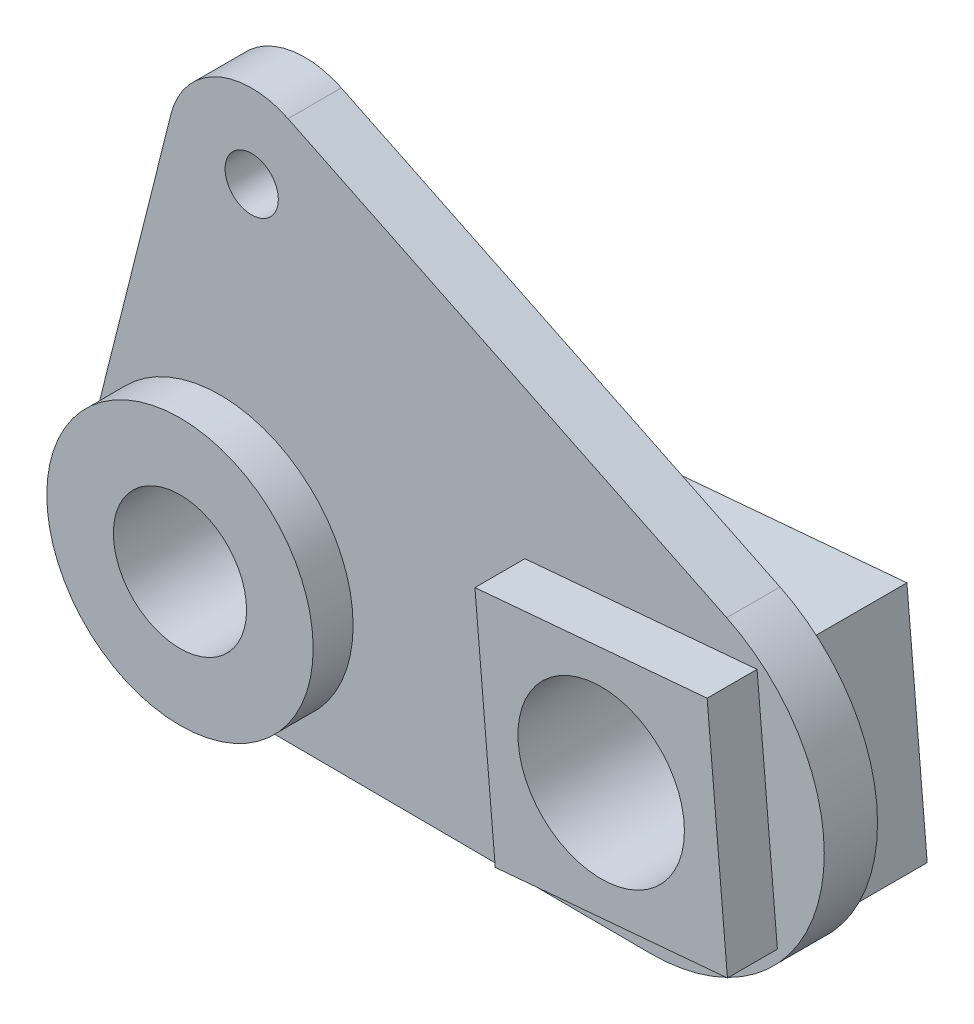
ISO-10303-21;
HEADER;
FILE_DESCRIPTION(('STEP AP214'),'2;1');
FILE_NAME('part.step','',(''),(''),'','','');
FILE_SCHEMA(('AUTOMOTIVE_DESIGN { 1 0 10303 214 1 1 1 1 }'));
ENDSEC;
DATA;
#1=APPLICATION_CONTEXT('core data for automotive mechanical design processes');
#2=APPLICATION_PROTOCOL_DEFINITION('international standard','automotive_design',2000,#1);
#3=PRODUCT_CONTEXT('',#1,'mechanical');
#4=PRODUCT('Part','Part','',(#3));
#5=PRODUCT_RELATED_PRODUCT_CATEGORY('part','',(#4));
#6=PRODUCT_DEFINITION_FORMATION('','',#4);
#7=PRODUCT_DEFINITION_CONTEXT('part definition',#1,'design');
#8=PRODUCT_DEFINITION('design','',#6,#7);
#9=PRODUCT_DEFINITION_SHAPE('','',#8);
#10=(LENGTH_UNIT() NAMED_UNIT(*) SI_UNIT(.MILLI.,.METRE.));
#11=(NAMED_UNIT(*) PLANE_ANGLE_UNIT() SI_UNIT($,.RADIAN.));
#12=(NAMED_UNIT(*) SI_UNIT($,.STERADIAN.) SOLID_ANGLE_UNIT());
#13=UNCERTAINTY_MEASURE_WITH_UNIT(LENGTH_MEASURE(1.E-05),#10,'distance_accuracy_value','');
#14=(GEOMETRIC_REPRESENTATION_CONTEXT(3) GLOBAL_UNCERTAINTY_ASSIGNED_CONTEXT((#13)) GLOBAL_UNIT_ASSIGNED_CONTEXT((#10,
#11,#12)) REPRESENTATION_CONTEXT('',''));
#15=CARTESIAN_POINT('',(0.,0.,0.));
#16=DIRECTION('',(0.,0.,1.));
#17=DIRECTION('',(1.,0.,0.));
#18=AXIS2_PLACEMENT_3D('',#15,#16,#17);
#19=CARTESIAN_POINT('',(0.,0.,20.));
#20=DIRECTION('',(0.,0.,1.));
#21=DIRECTION('',(1.,0.,0.));
#22=AXIS2_PLACEMENT_3D('',#19,#20,#21);
#23=PLANE('',#22);
#24=CARTESIAN_POINT('',(0.,0.,20.));
#25=DIRECTION('',(0.,0.,1.));
#26=DIRECTION('',(1.,0.,0.));
#27=AXIS2_PLACEMENT_3D('',#24,#25,#26);
#28=CIRCLE('',#27,40.);
#29=CARTESIAN_POINT('',(40.,0.,20.));
#30=VERTEX_POINT('',#29);
#31=EDGE_CURVE('E12',#30,#30,#28,.T.);
#32=ORIENTED_EDGE('',*,*,#31,.T.);
#33=EDGE_LOOP('',(#32));
#34=FACE_BOUND('',#33,.T.);
#35=CARTESIAN_POINT('',(0.,0.,20.));
#36=DIRECTION('',(0.,0.,1.));
#37=DIRECTION('',(1.,0.,0.));
#38=AXIS2_PLACEMENT_3D('',#35,#36,#37);
#39=CIRCLE('',#38,20.);
#40=CARTESIAN_POINT('',(20.,0.,20.));
#41=VERTEX_POINT('',#40);
#42=EDGE_CURVE('E301',#41,#41,#39,.T.);
#43=ORIENTED_EDGE('',*,*,#42,.F.);
#44=EDGE_LOOP('',(#43));
#45=FACE_BOUND('',#44,.T.);
#46=ADVANCED_FACE('F79',(#34,#45),#23,.T.);
#47=CARTESIAN_POINT('',(0.,0.,-20.));
#48=DIRECTION('',(0.,0.,1.));
#49=DIRECTION('',(1.,0.,0.));
#50=AXIS2_PLACEMENT_3D('',#47,#48,#49);
#51=PLANE('',#50);
#52=CARTESIAN_POINT('',(0.,0.,-20.));
#53=DIRECTION('',(0.,0.,1.));
#54=DIRECTION('',(1.,0.,0.));
#55=AXIS2_PLACEMENT_3D('',#52,#53,#54);
#56=CIRCLE('',#55,40.);
#57=CARTESIAN_POINT('',(40.,0.,-20.));
#58=VERTEX_POINT('',#57);
#59=EDGE_CURVE('E83',#58,#58,#56,.T.);
#60=ORIENTED_EDGE('',*,*,#59,.F.);
#61=EDGE_LOOP('',(#60));
#62=FACE_BOUND('',#61,.T.);
#63=CARTESIAN_POINT('',(0.,0.,-20.));
#64=DIRECTION('',(0.,0.,1.));
#65=DIRECTION('',(1.,0.,0.));
#66=AXIS2_PLACEMENT_3D('',#63,#64,#65);
#67=CIRCLE('',#66,20.);
#68=CARTESIAN_POINT('',(20.,0.,-20.));
#69=VERTEX_POINT('',#68);
#70=EDGE_CURVE('E305',#69,#69,#67,.T.);
#71=ORIENTED_EDGE('',*,*,#70,.T.);
#72=EDGE_LOOP('',(#71));
#73=FACE_BOUND('',#72,.T.);
#74=ADVANCED_FACE('F310',(#62,#73),#51,.F.);
#75=CARTESIAN_POINT('',(0.,0.,20.));
#76=DIRECTION('',(0.,0.,-1.));
#77=DIRECTION('',(-1.,0.,0.));
#78=AXIS2_PLACEMENT_3D('',#75,#76,#77);
#79=CYLINDRICAL_SURFACE('',#78,40.);
#80=CARTESIAN_POINT('',(0.,0.,8.));
#81=DIRECTION('',(0.,0.,1.));
#82=DIRECTION('',(1.,0.,0.));
#83=AXIS2_PLACEMENT_3D('',#80,#81,#82);
#84=CIRCLE('',#83,40.);
#85=CARTESIAN_POINT('',(-0.207064054868237,-39.9994640523743,8.));
#86=VERTEX_POINT('',#85);
#87=CARTESIAN_POINT('',(-38.7946049299003,9.74569793975542,8.));
#88=VERTEX_POINT('',#87);
#89=EDGE_CURVE('E96',#86,#88,#84,.T.);
#90=ORIENTED_EDGE('',*,*,#89,.T.);
#91=DIRECTION('',(0.,0.,-1.));
#92=VECTOR('',#91,1.);
#93=CARTESIAN_POINT('',(-38.7946049299003,9.74569793975542,8.));
#94=LINE('',#93,#92);
#95=CARTESIAN_POINT('',(-38.7946049299003,9.74569793975542,-8.));
#96=VERTEX_POINT('',#95);
#97=EDGE_CURVE('E288',#88,#96,#94,.T.);
#98=ORIENTED_EDGE('',*,*,#97,.T.);
#99=CARTESIAN_POINT('',(0.,0.,-8.));
#100=DIRECTION('',(0.,0.,1.));
#101=DIRECTION('',(1.,0.,0.));
#102=AXIS2_PLACEMENT_3D('',#99,#100,#101);
#103=CIRCLE('',#102,40.);
#104=CARTESIAN_POINT('',(-0.207064054868237,-39.9994640523743,-8.));
#105=VERTEX_POINT('',#104);
#106=EDGE_CURVE('E297',#105,#96,#103,.T.);
#107=ORIENTED_EDGE('',*,*,#106,.F.);
#108=DIRECTION('',(0.,0.,-1.));
#109=VECTOR('',#108,1.);
#110=CARTESIAN_POINT('',(-0.207064054868237,-39.9994640523743,8.));
#111=LINE('',#110,#109);
#112=EDGE_CURVE('E95',#86,#105,#111,.T.);
#113=ORIENTED_EDGE('',*,*,#112,.F.);
#114=EDGE_LOOP('',(#90,#98,#107,#113));
#115=FACE_BOUND('',#114,.T.);
#116=ORIENTED_EDGE('',*,*,#31,.F.);
#117=EDGE_LOOP('',(#116));
#118=FACE_BOUND('',#117,.T.);
#119=ORIENTED_EDGE('',*,*,#59,.T.);
#120=EDGE_LOOP('',(#119));
#121=FACE_BOUND('',#120,.T.);
#122=ADVANCED_FACE('F80',(#115,#118,#121),#79,.T.);
#123=CARTESIAN_POINT('',(0.,0.,20.));
#124=DIRECTION('',(0.,0.,-1.));
#125=DIRECTION('',(-1.,0.,0.));
#126=AXIS2_PLACEMENT_3D('',#123,#124,#125);
#127=CYLINDRICAL_SURFACE('',#126,20.);
#128=ORIENTED_EDGE('',*,*,#42,.T.);
#129=EDGE_LOOP('',(#128));
#130=FACE_BOUND('',#129,.T.);
#131=ORIENTED_EDGE('',*,*,#70,.F.);
#132=EDGE_LOOP('',(#131));
#133=FACE_BOUND('',#132,.T.);
#134=ADVANCED_FACE('F313',(#130,#133),#127,.F.);
#135=CARTESIAN_POINT('',(0.,0.,8.));
#136=DIRECTION('',(0.,0.,1.));
#137=DIRECTION('',(1.,0.,0.));
#138=AXIS2_PLACEMENT_3D('',#135,#136,#137);
#139=PLANE('',#138);
#140=CARTESIAN_POINT('',(9.54061085317714,99.5438433281951,8.));
#141=DIRECTION('',(0.,0.,1.));
#142=DIRECTION('',(1.,0.,0.));
#143=AXIS2_PLACEMENT_3D('',#140,#141,#142);
#144=CIRCLE('',#143,8.);
#145=CARTESIAN_POINT('',(17.5406108531771,99.5438433281951,8.));
#146=VERTEX_POINT('',#145);
#147=EDGE_CURVE('E245',#146,#146,#144,.T.);
#148=ORIENTED_EDGE('',*,*,#147,.F.);
#149=EDGE_LOOP('',(#148));
#150=FACE_BOUND('',#149,.T.);
#151=DIRECTION('',(0.087155742747652,-0.996194698091746,0.));
#152=VECTOR('',#151,1.);
#153=CARTESIAN_POINT('',(94.633185566789,8.27933093043853,8.));
#154=LINE('',#153,#152);
#155=CARTESIAN_POINT('',(91.5827345706211,43.1461453636503,8.));
#156=VERTEX_POINT('',#155);
#157=CARTESIAN_POINT('',(97.6836365629567,-26.587483502772,8.));
#158=VERTEX_POINT('',#157);
#159=EDGE_CURVE('E185',#156,#158,#154,.T.);
#160=ORIENTED_EDGE('',*,*,#159,.F.);
#161=DIRECTION('',(0.996194698091746,0.0871557427476584,0.));
#162=VECTOR('',#161,1.);
#163=CARTESIAN_POINT('',(-3.05045099616804,34.8668144332111,8.));
#164=LINE('',#163,#162);
#165=CARTESIAN_POINT('',(161.316363437043,49.2470473559863,8.));
#166=VERTEX_POINT('',#165);
#167=EDGE_CURVE('E237',#156,#166,#164,.T.);
#168=ORIENTED_EDGE('',*,*,#167,.T.);
#169=DIRECTION('',(-0.0871557427476524,0.996194698091746,0.));
#170=VECTOR('',#169,1.);
#171=CARTESIAN_POINT('',(164.366814433211,14.3802329227742,8.));
#172=LINE('',#171,#170);
#173=CARTESIAN_POINT('',(167.417265429379,-20.4865815104359,7.99999999999999));
#174=VERTEX_POINT('',#173);
#175=EDGE_CURVE('E239',#174,#166,#172,.T.);
#176=ORIENTED_EDGE('',*,*,#175,.F.);
#177=DIRECTION('',(0.996194698091746,0.0871557427476583,0.));
#178=VECTOR('',#177,1.);
#179=CARTESIAN_POINT('',(3.05045099616804,-34.8668144332111,8.));
#180=LINE('',#179,#178);
#181=EDGE_CURVE('E244',#158,#174,#180,.T.);
#182=ORIENTED_EDGE('',*,*,#181,.F.);
#183=EDGE_LOOP('',(#160,#168,#176,#182));
#184=FACE_BOUND('',#183,.T.);
#185=ORIENTED_EDGE('',*,*,#89,.F.);
#186=DIRECTION('',(0.999986601309357,-0.00517660137170592,0.));
#187=VECTOR('',#186,1.);
#188=CARTESIAN_POINT('',(-0.207064054868237,-39.9994640523743,8.));
#189=LINE('',#188,#187);
#190=CARTESIAN_POINT('',(129.230816728671,-40.6695213414794,8.));
#191=VERTEX_POINT('',#190);
#192=EDGE_CURVE('E250',#86,#191,#189,.T.);
#193=ORIENTED_EDGE('',*,*,#192,.T.);
#194=CARTESIAN_POINT('',(129.5,11.3297819266072,8.));
#195=DIRECTION('',(0.,0.,1.));
#196=DIRECTION('',(1.,0.,0.));
#197=AXIS2_PLACEMENT_3D('',#194,#195,#196);
#198=CIRCLE('',#197,52.);
#199=CARTESIAN_POINT('',(152.199371640368,58.1137377996674,8.));
#200=VERTEX_POINT('',#199);
#201=EDGE_CURVE('E249',#191,#200,#198,.T.);
#202=ORIENTED_EDGE('',*,*,#201,.T.);
#203=DIRECTION('',(0.899691459097311,-0.436526377699392,0.));
#204=VECTOR('',#203,1.);
#205=CARTESIAN_POINT('',(51.8259280290443,106.814495502566,8.));
#206=LINE('',#205,#204);
#207=CARTESIAN_POINT('',(20.453770295662,122.036129805628,8.));
#208=VERTEX_POINT('',#207);
#209=EDGE_CURVE('E252',#208,#200,#206,.T.);
#210=ORIENTED_EDGE('',*,*,#209,.F.);
#211=CARTESIAN_POINT('',(9.54061085317714,99.5438433281951,8.));
#212=DIRECTION('',(0.,0.,1.));
#213=DIRECTION('',(1.,0.,0.));
#214=AXIS2_PLACEMENT_3D('',#211,#212,#213);
#215=CIRCLE('',#214,25.);
#216=CARTESIAN_POINT('',(-14.7060172280106,105.634904540542,8.));
#217=VERTEX_POINT('',#216);
#218=EDGE_CURVE('E254',#208,#217,#215,.T.);
#219=ORIENTED_EDGE('',*,*,#218,.T.);
#220=DIRECTION('',(-0.243642448493885,-0.969865123247508,0.));
#221=VECTOR('',#220,1.);
#222=CARTESIAN_POINT('',(-38.7946049299003,9.74569793975542,8.));
#223=LINE('',#222,#221);
#224=EDGE_CURVE('E260',#217,#88,#223,.T.);
#225=ORIENTED_EDGE('',*,*,#224,.T.);
#226=EDGE_LOOP('',(#185,#193,#202,#210,#219,#225));
#227=FACE_BOUND('',#226,.T.);
#228=ADVANCED_FACE('F311',(#150,#184,#227),#139,.T.);
#229=CARTESIAN_POINT('',(0.,0.,-8.));
#230=DIRECTION('',(0.,0.,1.));
#231=DIRECTION('',(1.,0.,0.));
#232=AXIS2_PLACEMENT_3D('',#229,#230,#231);
#233=PLANE('',#232);
#234=CARTESIAN_POINT('',(9.54061085317714,99.5438433281951,-8.));
#235=DIRECTION('',(0.,0.,1.));
#236=DIRECTION('',(1.,0.,0.));
#237=AXIS2_PLACEMENT_3D('',#234,#235,#236);
#238=CIRCLE('',#237,8.);
#239=CARTESIAN_POINT('',(17.5406108531771,99.5438433281951,-8.));
#240=VERTEX_POINT('',#239);
#241=EDGE_CURVE('E267',#240,#240,#238,.T.);
#242=ORIENTED_EDGE('',*,*,#241,.T.);
#243=EDGE_LOOP('',(#242));
#244=FACE_BOUND('',#243,.T.);
#245=DIRECTION('',(0.087155742747652,-0.996194698091746,0.));
#246=VECTOR('',#245,1.);
#247=CARTESIAN_POINT('',(94.633185566789,8.27933093043853,-8.));
#248=LINE('',#247,#246);
#249=CARTESIAN_POINT('',(91.5827345706211,43.1461453636503,-8.00000000000001));
#250=VERTEX_POINT('',#249);
#251=CARTESIAN_POINT('',(97.6836365629567,-26.587483502772,-8.00000000000001));
#252=VERTEX_POINT('',#251);
#253=EDGE_CURVE('E228',#250,#252,#248,.T.);
#254=ORIENTED_EDGE('',*,*,#253,.T.);
#255=DIRECTION('',(0.996194698091746,0.0871557427476583,0.));
#256=VECTOR('',#255,1.);
#257=CARTESIAN_POINT('',(3.05045099616804,-34.8668144332111,-8.));
#258=LINE('',#257,#256);
#259=CARTESIAN_POINT('',(167.417265429379,-20.4865815104359,-8.));
#260=VERTEX_POINT('',#259);
#261=EDGE_CURVE('E266',#252,#260,#258,.T.);
#262=ORIENTED_EDGE('',*,*,#261,.T.);
#263=DIRECTION('',(-0.0871557427476524,0.996194698091746,0.));
#264=VECTOR('',#263,1.);
#265=CARTESIAN_POINT('',(164.366814433211,14.3802329227742,-8.));
#266=LINE('',#265,#264);
#267=CARTESIAN_POINT('',(161.316363437043,49.2470473559863,-8.00000000000001));
#268=VERTEX_POINT('',#267);
#269=EDGE_CURVE('E263',#260,#268,#266,.T.);
#270=ORIENTED_EDGE('',*,*,#269,.T.);
#271=DIRECTION('',(0.996194698091746,0.0871557427476584,0.));
#272=VECTOR('',#271,1.);
#273=CARTESIAN_POINT('',(-3.05045099616804,34.8668144332111,-8.));
#274=LINE('',#273,#272);
#275=EDGE_CURVE('E261',#250,#268,#274,.T.);
#276=ORIENTED_EDGE('',*,*,#275,.F.);
#277=EDGE_LOOP('',(#254,#262,#270,#276));
#278=FACE_BOUND('',#277,.T.);
#279=DIRECTION('',(0.999986601309357,-0.00517660137170592,0.));
#280=VECTOR('',#279,1.);
#281=CARTESIAN_POINT('',(-0.207064054868237,-39.9994640523743,-8.));
#282=LINE('',#281,#280);
#283=CARTESIAN_POINT('',(129.230816728671,-40.6695213414794,-8.));
#284=VERTEX_POINT('',#283);
#285=EDGE_CURVE('E275',#105,#284,#282,.T.);
#286=ORIENTED_EDGE('',*,*,#285,.F.);
#287=ORIENTED_EDGE('',*,*,#106,.T.);
#288=DIRECTION('',(-0.243642448493885,-0.969865123247508,0.));
#289=VECTOR('',#288,1.);
#290=CARTESIAN_POINT('',(-38.7946049299003,9.74569793975542,-8.));
#291=LINE('',#290,#289);
#292=CARTESIAN_POINT('',(-14.7060172280106,105.634904540542,-8.));
#293=VERTEX_POINT('',#292);
#294=EDGE_CURVE('E240',#293,#96,#291,.T.);
#295=ORIENTED_EDGE('',*,*,#294,.F.);
#296=CARTESIAN_POINT('',(9.54061085317714,99.5438433281951,-8.));
#297=DIRECTION('',(0.,0.,1.));
#298=DIRECTION('',(1.,0.,0.));
#299=AXIS2_PLACEMENT_3D('',#296,#297,#298);
#300=CIRCLE('',#299,25.);
#301=CARTESIAN_POINT('',(20.453770295662,122.036129805628,-8.));
#302=VERTEX_POINT('',#301);
#303=EDGE_CURVE('E283',#302,#293,#300,.T.);
#304=ORIENTED_EDGE('',*,*,#303,.F.);
#305=DIRECTION('',(0.899691459097311,-0.436526377699392,0.));
#306=VECTOR('',#305,1.);
#307=CARTESIAN_POINT('',(51.8259280290443,106.814495502566,-8.));
#308=LINE('',#307,#306);
#309=CARTESIAN_POINT('',(152.199371640368,58.1137377996674,-8.));
#310=VERTEX_POINT('',#309);
#311=EDGE_CURVE('E279',#302,#310,#308,.T.);
#312=ORIENTED_EDGE('',*,*,#311,.T.);
#313=CARTESIAN_POINT('',(129.5,11.3297819266072,-8.));
#314=DIRECTION('',(0.,0.,1.));
#315=DIRECTION('',(1.,0.,0.));
#316=AXIS2_PLACEMENT_3D('',#313,#314,#315);
#317=CIRCLE('',#316,52.);
#318=EDGE_CURVE('E274',#284,#310,#317,.T.);
#319=ORIENTED_EDGE('',*,*,#318,.F.);
#320=EDGE_LOOP('',(#286,#287,#295,#304,#312,#319));
#321=FACE_BOUND('',#320,.T.);
#322=ADVANCED_FACE('F319',(#244,#278,#321),#233,.F.);
#323=CARTESIAN_POINT('',(-0.207064054868237,-39.9994640523743,8.));
#324=DIRECTION('',(0.00517660137170592,0.999986601309357,0.));
#325=DIRECTION('',(-0.999986601309357,0.00517660137170592,0.));
#326=AXIS2_PLACEMENT_3D('',#323,#324,#325);
#327=PLANE('',#326);
#328=ORIENTED_EDGE('',*,*,#285,.T.);
#329=DIRECTION('',(0.,0.,-1.));
#330=VECTOR('',#329,1.);
#331=CARTESIAN_POINT('',(129.230816728671,-40.6695213414794,8.));
#332=LINE('',#331,#330);
#333=EDGE_CURVE('E293',#191,#284,#332,.T.);
#334=ORIENTED_EDGE('',*,*,#333,.F.);
#335=ORIENTED_EDGE('',*,*,#192,.F.);
#336=ORIENTED_EDGE('',*,*,#112,.T.);
#337=EDGE_LOOP('',(#328,#334,#335,#336));
#338=FACE_BOUND('',#337,.T.);
#339=ADVANCED_FACE('F364',(#338),#327,.F.);
#340=CARTESIAN_POINT('',(129.5,11.3297819266072,8.));
#341=DIRECTION('',(0.,0.,-1.));
#342=DIRECTION('',(-1.,0.,0.));
#343=AXIS2_PLACEMENT_3D('',#340,#341,#342);
#344=CYLINDRICAL_SURFACE('',#343,52.);
#345=ORIENTED_EDGE('',*,*,#318,.T.);
#346=DIRECTION('',(0.,0.,-1.));
#347=VECTOR('',#346,1.);
#348=CARTESIAN_POINT('',(152.199371640368,58.1137377996674,8.));
#349=LINE('',#348,#347);
#350=EDGE_CURVE('E291',#200,#310,#349,.T.);
#351=ORIENTED_EDGE('',*,*,#350,.F.);
#352=ORIENTED_EDGE('',*,*,#201,.F.);
#353=ORIENTED_EDGE('',*,*,#333,.T.);
#354=EDGE_LOOP('',(#345,#351,#352,#353));
#355=FACE_BOUND('',#354,.T.);
#356=ADVANCED_FACE('F376',(#355),#344,.T.);
#357=CARTESIAN_POINT('',(51.8259280290443,106.814495502566,8.));
#358=DIRECTION('',(0.436526377699392,0.899691459097311,0.));
#359=DIRECTION('',(-0.899691459097311,0.436526377699392,0.));
#360=AXIS2_PLACEMENT_3D('',#357,#358,#359);
#361=PLANE('',#360);
#362=ORIENTED_EDGE('',*,*,#311,.F.);
#363=DIRECTION('',(0.,0.,-1.));
#364=VECTOR('',#363,1.);
#365=CARTESIAN_POINT('',(20.453770295662,122.036129805628,8.));
#366=LINE('',#365,#364);
#367=EDGE_CURVE('E292',#208,#302,#366,.T.);
#368=ORIENTED_EDGE('',*,*,#367,.F.);
#369=ORIENTED_EDGE('',*,*,#209,.T.);
#370=ORIENTED_EDGE('',*,*,#350,.T.);
#371=EDGE_LOOP('',(#362,#368,#369,#370));
#372=FACE_BOUND('',#371,.T.);
#373=ADVANCED_FACE('F387',(#372),#361,.T.);
#374=CARTESIAN_POINT('',(9.54061085317714,99.5438433281951,8.));
#375=DIRECTION('',(0.,0.,-1.));
#376=DIRECTION('',(-1.,0.,0.));
#377=AXIS2_PLACEMENT_3D('',#374,#375,#376);
#378=CYLINDRICAL_SURFACE('',#377,25.);
#379=ORIENTED_EDGE('',*,*,#303,.T.);
#380=DIRECTION('',(0.,0.,-1.));
#381=VECTOR('',#380,1.);
#382=CARTESIAN_POINT('',(-14.7060172280106,105.634904540542,8.));
#383=LINE('',#382,#381);
#384=EDGE_CURVE('E286',#217,#293,#383,.T.);
#385=ORIENTED_EDGE('',*,*,#384,.F.);
#386=ORIENTED_EDGE('',*,*,#218,.F.);
#387=ORIENTED_EDGE('',*,*,#367,.T.);
#388=EDGE_LOOP('',(#379,#385,#386,#387));
#389=FACE_BOUND('',#388,.T.);
#390=ADVANCED_FACE('F398',(#389),#378,.T.);
#391=CARTESIAN_POINT('',(-38.7946049299003,9.74569793975542,8.));
#392=DIRECTION('',(0.969865123247508,-0.243642448493885,0.));
#393=DIRECTION('',(0.243642448493885,0.969865123247508,0.));
#394=AXIS2_PLACEMENT_3D('',#391,#392,#393);
#395=PLANE('',#394);
#396=ORIENTED_EDGE('',*,*,#294,.T.);
#397=ORIENTED_EDGE('',*,*,#97,.F.);
#398=ORIENTED_EDGE('',*,*,#224,.F.);
#399=ORIENTED_EDGE('',*,*,#384,.T.);
#400=EDGE_LOOP('',(#396,#397,#398,#399));
#401=FACE_BOUND('',#400,.T.);
#402=ADVANCED_FACE('F408',(#401),#395,.F.);
#403=CARTESIAN_POINT('',(9.54061085317714,99.5438433281951,8.));
#404=DIRECTION('',(0.,0.,-1.));
#405=DIRECTION('',(-1.,0.,0.));
#406=AXIS2_PLACEMENT_3D('',#403,#404,#405);
#407=CYLINDRICAL_SURFACE('',#406,8.);
#408=ORIENTED_EDGE('',*,*,#147,.T.);
#409=EDGE_LOOP('',(#408));
#410=FACE_BOUND('',#409,.T.);
#411=ORIENTED_EDGE('',*,*,#241,.F.);
#412=EDGE_LOOP('',(#411));
#413=FACE_BOUND('',#412,.T.);
#414=ADVANCED_FACE('F418',(#410,#413),#407,.F.);
#415=CARTESIAN_POINT('',(-3.05045099616804,34.8668144332111,-37.));
#416=DIRECTION('',(-0.0871557427476582,0.996194698091745,0.));
#417=DIRECTION('',(-0.996194698091746,-0.0871557427476582,0.));
#418=AXIS2_PLACEMENT_3D('',#415,#416,#417);
#419=PLANE('',#418);
#420=ORIENTED_EDGE('',*,*,#275,.T.);
#421=DIRECTION('',(0.,0.,1.));
#422=VECTOR('',#421,1.);
#423=CARTESIAN_POINT('',(161.316363437043,49.2470473559863,-37.));
#424=LINE('',#423,#422);
#425=CARTESIAN_POINT('',(161.316363437043,49.2470473559863,-37.));
#426=VERTEX_POINT('',#425);
#427=EDGE_CURVE('E227',#426,#268,#424,.T.);
#428=ORIENTED_EDGE('',*,*,#427,.F.);
#429=DIRECTION('',(-0.996194698091746,-0.0871557427476582,0.));
#430=VECTOR('',#429,1.);
#431=CARTESIAN_POINT('',(-3.05045099616804,34.8668144332111,-37.));
#432=LINE('',#431,#430);
#433=CARTESIAN_POINT('',(91.5827345706211,43.1461453636503,-37.));
#434=VERTEX_POINT('',#433);
#435=EDGE_CURVE('E189',#426,#434,#432,.T.);
#436=ORIENTED_EDGE('',*,*,#435,.T.);
#437=DIRECTION('',(0.,0.,1.));
#438=VECTOR('',#437,1.);
#439=CARTESIAN_POINT('',(91.5827345706211,43.1461453636503,-37.));
#440=LINE('',#439,#438);
#441=EDGE_CURVE('E224',#434,#250,#440,.T.);
#442=ORIENTED_EDGE('',*,*,#441,.T.);
#443=EDGE_LOOP('',(#420,#428,#436,#442));
#444=FACE_BOUND('',#443,.T.);
#445=ADVANCED_FACE('F426',(#444),#419,.T.);
#446=CARTESIAN_POINT('',(3.05045099616805,-34.8668144332111,-37.));
#447=DIRECTION('',(-0.0871557427476585,0.996194698091745,0.));
#448=DIRECTION('',(-0.996194698091746,-0.0871557427476585,0.));
#449=AXIS2_PLACEMENT_3D('',#446,#447,#448);
#450=PLANE('',#449);
#451=DIRECTION('',(0.,0.,1.));
#452=VECTOR('',#451,1.);
#453=CARTESIAN_POINT('',(167.417265429379,-20.4865815104359,-37.));
#454=LINE('',#453,#452);
#455=CARTESIAN_POINT('',(167.417265429379,-20.4865815104359,-37.));
#456=VERTEX_POINT('',#455);
#457=EDGE_CURVE('E235',#456,#260,#454,.T.);
#458=ORIENTED_EDGE('',*,*,#457,.T.);
#459=ORIENTED_EDGE('',*,*,#261,.F.);
#460=DIRECTION('',(0.,0.,1.));
#461=VECTOR('',#460,1.);
#462=CARTESIAN_POINT('',(97.6836365629567,-26.587483502772,-37.));
#463=LINE('',#462,#461);
#464=CARTESIAN_POINT('',(97.6836365629567,-26.587483502772,-37.));
#465=VERTEX_POINT('',#464);
#466=EDGE_CURVE('E188',#465,#252,#463,.T.);
#467=ORIENTED_EDGE('',*,*,#466,.F.);
#468=DIRECTION('',(-0.996194698091746,-0.0871557427476585,0.));
#469=VECTOR('',#468,1.);
#470=CARTESIAN_POINT('',(3.05045099616805,-34.8668144332111,-37.));
#471=LINE('',#470,#469);
#472=EDGE_CURVE('E216',#456,#465,#471,.T.);
#473=ORIENTED_EDGE('',*,*,#472,.F.);
#474=EDGE_LOOP('',(#458,#459,#467,#473));
#475=FACE_BOUND('',#474,.T.);
#476=ADVANCED_FACE('F434',(#475),#450,.F.);
#477=CARTESIAN_POINT('',(94.6331855667889,8.27933093043856,-37.));
#478=DIRECTION('',(-0.996194698091746,-0.0871557427476523,0.));
#479=DIRECTION('',(0.0871557427476523,-0.996194698091746,0.));
#480=AXIS2_PLACEMENT_3D('',#477,#478,#479);
#481=PLANE('',#480);
#482=ORIENTED_EDGE('',*,*,#253,.F.);
#483=ORIENTED_EDGE('',*,*,#441,.F.);
#484=DIRECTION('',(0.0871557427476523,-0.996194698091746,0.));
#485=VECTOR('',#484,1.);
#486=CARTESIAN_POINT('',(94.6331855667889,8.27933093043856,-37.));
#487=LINE('',#486,#485);
#488=EDGE_CURVE('E213',#434,#465,#487,.T.);
#489=ORIENTED_EDGE('',*,*,#488,.T.);
#490=ORIENTED_EDGE('',*,*,#466,.T.);
#491=EDGE_LOOP('',(#482,#483,#489,#490));
#492=FACE_BOUND('',#491,.T.);
#493=ADVANCED_FACE('F449',(#492),#481,.T.);
#494=CARTESIAN_POINT('',(164.366814433211,14.3802329227743,-37.));
#495=DIRECTION('',(0.996194698091746,0.0871557427476527,0.));
#496=DIRECTION('',(-0.0871557427476527,0.996194698091746,0.));
#497=AXIS2_PLACEMENT_3D('',#494,#495,#496);
#498=PLANE('',#497);
#499=ORIENTED_EDGE('',*,*,#269,.F.);
#500=ORIENTED_EDGE('',*,*,#457,.F.);
#501=DIRECTION('',(-0.0871557427476527,0.996194698091746,0.));
#502=VECTOR('',#501,1.);
#503=CARTESIAN_POINT('',(164.366814433211,14.3802329227743,-37.));
#504=LINE('',#503,#502);
#505=EDGE_CURVE('E217',#456,#426,#504,.T.);
#506=ORIENTED_EDGE('',*,*,#505,.T.);
#507=ORIENTED_EDGE('',*,*,#427,.T.);
#508=EDGE_LOOP('',(#499,#500,#506,#507));
#509=FACE_BOUND('',#508,.T.);
#510=ADVANCED_FACE('F460',(#509),#498,.T.);
#511=CARTESIAN_POINT('',(91.5827345706211,43.1461453636503,23.));
#512=VERTEX_POINT('',#511);
#513=EDGE_CURVE('E229',#156,#512,#440,.T.);
#514=ORIENTED_EDGE('',*,*,#513,.F.);
#515=ORIENTED_EDGE('',*,*,#159,.T.);
#516=CARTESIAN_POINT('',(97.6836365629567,-26.587483502772,23.));
#517=VERTEX_POINT('',#516);
#518=EDGE_CURVE('E180',#158,#517,#463,.T.);
#519=ORIENTED_EDGE('',*,*,#518,.T.);
#520=DIRECTION('',(0.0871557427476523,-0.996194698091746,0.));
#521=VECTOR('',#520,1.);
#522=CARTESIAN_POINT('',(94.6331855667889,8.27933093043856,23.));
#523=LINE('',#522,#521);
#524=EDGE_CURVE('E182',#512,#517,#523,.T.);
#525=ORIENTED_EDGE('',*,*,#524,.F.);
#526=EDGE_LOOP('',(#514,#515,#519,#525));
#527=FACE_BOUND('',#526,.T.);
#528=ADVANCED_FACE('F179',(#527),#481,.T.);
#529=CARTESIAN_POINT('',(161.316363437043,49.2470473559863,23.));
#530=VERTEX_POINT('',#529);
#531=EDGE_CURVE('E233',#166,#530,#424,.T.);
#532=ORIENTED_EDGE('',*,*,#531,.F.);
#533=ORIENTED_EDGE('',*,*,#167,.F.);
#534=ORIENTED_EDGE('',*,*,#513,.T.);
#535=DIRECTION('',(-0.996194698091746,-0.0871557427476582,0.));
#536=VECTOR('',#535,1.);
#537=CARTESIAN_POINT('',(-3.05045099616804,34.8668144332111,23.));
#538=LINE('',#537,#536);
#539=EDGE_CURVE('E197',#530,#512,#538,.T.);
#540=ORIENTED_EDGE('',*,*,#539,.F.);
#541=EDGE_LOOP('',(#532,#533,#534,#540));
#542=FACE_BOUND('',#541,.T.);
#543=ADVANCED_FACE('F437',(#542),#419,.T.);
#544=CARTESIAN_POINT('',(167.417265429379,-20.4865815104359,23.));
#545=VERTEX_POINT('',#544);
#546=EDGE_CURVE('E205',#174,#545,#454,.T.);
#547=ORIENTED_EDGE('',*,*,#546,.F.);
#548=ORIENTED_EDGE('',*,*,#175,.T.);
#549=ORIENTED_EDGE('',*,*,#531,.T.);
#550=DIRECTION('',(-0.0871557427476527,0.996194698091746,0.));
#551=VECTOR('',#550,1.);
#552=CARTESIAN_POINT('',(164.366814433211,14.3802329227743,23.));
#553=LINE('',#552,#551);
#554=EDGE_CURVE('E204',#545,#530,#553,.T.);
#555=ORIENTED_EDGE('',*,*,#554,.F.);
#556=EDGE_LOOP('',(#547,#548,#549,#555));
#557=FACE_BOUND('',#556,.T.);
#558=ADVANCED_FACE('F467',(#557),#498,.T.);
#559=ORIENTED_EDGE('',*,*,#181,.T.);
#560=ORIENTED_EDGE('',*,*,#546,.T.);
#561=DIRECTION('',(-0.996194698091746,-0.0871557427476585,0.));
#562=VECTOR('',#561,1.);
#563=CARTESIAN_POINT('',(3.05045099616805,-34.8668144332111,23.));
#564=LINE('',#563,#562);
#565=EDGE_CURVE('E194',#545,#517,#564,.T.);
#566=ORIENTED_EDGE('',*,*,#565,.T.);
#567=ORIENTED_EDGE('',*,*,#518,.F.);
#568=EDGE_LOOP('',(#559,#560,#566,#567));
#569=FACE_BOUND('',#568,.T.);
#570=ADVANCED_FACE('F199',(#569),#450,.F.);
#571=CARTESIAN_POINT('',(0.,0.,-37.));
#572=DIRECTION('',(0.,0.,-1.));
#573=DIRECTION('',(-1.,0.,0.));
#574=AXIS2_PLACEMENT_3D('',#571,#572,#573);
#575=PLANE('',#574);
#576=CARTESIAN_POINT('',(129.5,11.3297819266072,-37.));
#577=DIRECTION('',(0.,0.,1.));
#578=DIRECTION('',(1.,0.,0.));
#579=AXIS2_PLACEMENT_3D('',#576,#577,#578);
#580=CIRCLE('',#579,25.);
#581=CARTESIAN_POINT('',(154.5,11.3297819266072,-37.));
#582=VERTEX_POINT('',#581);
#583=EDGE_CURVE('E209',#582,#582,#580,.T.);
#584=ORIENTED_EDGE('',*,*,#583,.T.);
#585=EDGE_LOOP('',(#584));
#586=FACE_BOUND('',#585,.T.);
#587=ORIENTED_EDGE('',*,*,#488,.F.);
#588=ORIENTED_EDGE('',*,*,#435,.F.);
#589=ORIENTED_EDGE('',*,*,#505,.F.);
#590=ORIENTED_EDGE('',*,*,#472,.T.);
#591=EDGE_LOOP('',(#587,#588,#589,#590));
#592=FACE_BOUND('',#591,.T.);
#593=ADVANCED_FACE('F498',(#586,#592),#575,.T.);
#594=CARTESIAN_POINT('',(129.5,11.3297819266072,-37.));
#595=DIRECTION('',(0.,0.,1.));
#596=DIRECTION('',(1.,0.,0.));
#597=AXIS2_PLACEMENT_3D('',#594,#595,#596);
#598=CYLINDRICAL_SURFACE('',#597,25.);
#599=CARTESIAN_POINT('',(129.5,11.3297819266072,23.));
#600=DIRECTION('',(0.,0.,1.));
#601=DIRECTION('',(1.,0.,0.));
#602=AXIS2_PLACEMENT_3D('',#599,#600,#601);
#603=CIRCLE('',#602,25.);
#604=CARTESIAN_POINT('',(154.5,11.3297819266072,23.));
#605=VERTEX_POINT('',#604);
#606=EDGE_CURVE('E196',#605,#605,#603,.T.);
#607=CARTESIAN_POINT('',(154.5,11.3297819266072,-37.));
#608=CARTESIAN_POINT('',(154.5,11.3297819266072,-36.375));
#609=CARTESIAN_POINT('',(154.5,11.3297819266072,-35.75));
#610=CARTESIAN_POINT('',(154.5,11.3297819266072,-34.5));
#611=CARTESIAN_POINT('',(154.5,11.3297819266072,-33.875));
#612=CARTESIAN_POINT('',(154.5,11.3297819266072,-32.625));
#613=CARTESIAN_POINT('',(154.5,11.3297819266072,-32.));
#614=CARTESIAN_POINT('',(154.5,11.3297819266072,-30.75));
#615=CARTESIAN_POINT('',(154.5,11.3297819266072,-30.125));
#616=CARTESIAN_POINT('',(154.5,11.3297819266072,-28.875));
#617=CARTESIAN_POINT('',(154.5,11.3297819266072,-28.25));
#618=CARTESIAN_POINT('',(154.5,11.3297819266072,-27.));
#619=CARTESIAN_POINT('',(154.5,11.3297819266072,-26.375));
#620=CARTESIAN_POINT('',(154.5,11.3297819266072,-25.125));
#621=CARTESIAN_POINT('',(154.5,11.3297819266072,-24.5));
#622=CARTESIAN_POINT('',(154.5,11.3297819266072,-23.25));
#623=CARTESIAN_POINT('',(154.5,11.3297819266072,-22.625));
#624=CARTESIAN_POINT('',(154.5,11.3297819266072,-21.375));
#625=CARTESIAN_POINT('',(154.5,11.3297819266072,-20.75));
#626=CARTESIAN_POINT('',(154.5,11.3297819266072,-19.5));
#627=CARTESIAN_POINT('',(154.5,11.3297819266072,-18.875));
#628=CARTESIAN_POINT('',(154.5,11.3297819266072,-17.625));
#629=CARTESIAN_POINT('',(154.5,11.3297819266072,-17.));
#630=CARTESIAN_POINT('',(154.5,11.3297819266072,-15.75));
#631=CARTESIAN_POINT('',(154.5,11.3297819266072,-15.125));
#632=CARTESIAN_POINT('',(154.5,11.3297819266072,-13.875));
#633=CARTESIAN_POINT('',(154.5,11.3297819266072,-13.25));
#634=CARTESIAN_POINT('',(154.5,11.3297819266072,-12.));
#635=CARTESIAN_POINT('',(154.5,11.3297819266072,-11.375));
#636=CARTESIAN_POINT('',(154.5,11.3297819266072,-10.125));
#637=CARTESIAN_POINT('',(154.5,11.3297819266072,-9.5));
#638=CARTESIAN_POINT('',(154.5,11.3297819266072,-8.25));
#639=CARTESIAN_POINT('',(154.5,11.3297819266072,-7.625));
#640=CARTESIAN_POINT('',(154.5,11.3297819266072,-6.37500000000001));
#641=CARTESIAN_POINT('',(154.5,11.3297819266072,-5.75000000000001));
#642=CARTESIAN_POINT('',(154.5,11.3297819266072,-4.50000000000001));
#643=CARTESIAN_POINT('',(154.5,11.3297819266072,-3.87500000000001));
#644=CARTESIAN_POINT('',(154.5,11.3297819266072,-2.62500000000001));
#645=CARTESIAN_POINT('',(154.5,11.3297819266072,-2.00000000000001));
#646=CARTESIAN_POINT('',(154.5,11.3297819266072,-0.750000000000008));
#647=CARTESIAN_POINT('',(154.5,11.3297819266072,-0.125000000000007));
#648=CARTESIAN_POINT('',(154.5,11.3297819266072,1.12499999999999));
#649=CARTESIAN_POINT('',(154.5,11.3297819266072,1.74999999999999));
#650=CARTESIAN_POINT('',(154.5,11.3297819266072,2.99999999999999));
#651=CARTESIAN_POINT('',(154.5,11.3297819266072,3.62499999999999));
#652=CARTESIAN_POINT('',(154.5,11.3297819266072,4.87499999999999));
#653=CARTESIAN_POINT('',(154.5,11.3297819266072,5.49999999999999));
#654=CARTESIAN_POINT('',(154.5,11.3297819266072,6.74999999999999));
#655=CARTESIAN_POINT('',(154.5,11.3297819266072,7.37499999999999));
#656=CARTESIAN_POINT('',(154.5,11.3297819266072,8.62499999999999));
#657=CARTESIAN_POINT('',(154.5,11.3297819266072,9.24999999999999));
#658=CARTESIAN_POINT('',(154.5,11.3297819266072,10.5));
#659=CARTESIAN_POINT('',(154.5,11.3297819266072,11.125));
#660=CARTESIAN_POINT('',(154.5,11.3297819266072,12.375));
#661=CARTESIAN_POINT('',(154.5,11.3297819266072,13.));
#662=CARTESIAN_POINT('',(154.5,11.3297819266072,14.25));
#663=CARTESIAN_POINT('',(154.5,11.3297819266072,14.875));
#664=CARTESIAN_POINT('',(154.5,11.3297819266072,16.125));
#665=CARTESIAN_POINT('',(154.5,11.3297819266072,16.75));
#666=CARTESIAN_POINT('',(154.5,11.3297819266072,18.));
#667=CARTESIAN_POINT('',(154.5,11.3297819266072,18.625));
#668=CARTESIAN_POINT('',(154.5,11.3297819266072,19.875));
#669=CARTESIAN_POINT('',(154.5,11.3297819266072,20.5));
#670=CARTESIAN_POINT('',(154.5,11.3297819266072,21.75));
#671=CARTESIAN_POINT('',(154.5,11.3297819266072,22.375));
#672=CARTESIAN_POINT('',(154.5,11.3297819266072,23.));
#673=B_SPLINE_CURVE_WITH_KNOTS('',3,(#607,#608,#609,#610,#611,#612,#613,#614,#615,#616,#617,
#618,#619,#620,#621,#622,#623,#624,#625,#626,#627,#628,#629,#630,#631,#632,#633,#634,#635,#636,
#637,#638,#639,#640,#641,#642,#643,#644,#645,#646,#647,#648,#649,#650,#651,#652,#653,#654,#655,
#656,#657,#658,#659,#660,#661,#662,#663,#664,#665,#666,#667,#668,#669,#670,#671,#672),
.UNSPECIFIED.,.F.,.F.,(4,2,2,2,2,2,2,2,2,2,2,2,2,2,2,2,2,2,2,2,2,2,2,2,2,2,2,2,2,2,2,2,4),(0.,
1.875,3.75,5.62500000000001,7.5,9.375,11.25,13.125,15.,16.875,18.75,20.625,22.5,24.375,26.25,
28.125,30.,31.875,33.75,35.625,37.5,39.375,41.25,43.125,45.,46.875,48.75,50.625,52.5,54.375,
56.25,58.125,60.),.UNSPECIFIED.);
#674=EDGE_CURVE('BSEAM510',#582,#605,#673,.T.);
#675=ORIENTED_EDGE('',*,*,#583,.F.);
#676=ORIENTED_EDGE('',*,*,#606,.T.);
#677=ORIENTED_EDGE('',*,*,#674,.T.);
#678=ORIENTED_EDGE('',*,*,#674,.F.);
#679=EDGE_LOOP('',(#675,#677,#676,#678));
#680=FACE_BOUND('',#679,.T.);
#681=ADVANCED_FACE('F510',(#680),#598,.F.);
#682=CARTESIAN_POINT('',(0.,0.,23.));
#683=DIRECTION('',(0.,0.,-1.));
#684=DIRECTION('',(-1.,0.,0.));
#685=AXIS2_PLACEMENT_3D('',#682,#683,#684);
#686=PLANE('',#685);
#687=ORIENTED_EDGE('',*,*,#524,.T.);
#688=ORIENTED_EDGE('',*,*,#565,.F.);
#689=ORIENTED_EDGE('',*,*,#554,.T.);
#690=ORIENTED_EDGE('',*,*,#539,.T.);
#691=EDGE_LOOP('',(#687,#688,#689,#690));
#692=FACE_BOUND('',#691,.T.);
#693=ORIENTED_EDGE('',*,*,#606,.F.);
#694=EDGE_LOOP('',(#693));
#695=FACE_BOUND('',#694,.T.);
#696=ADVANCED_FACE('F195',(#692,#695),#686,.F.);
#697=CLOSED_SHELL('',(#46,#74,#122,#134,#228,#322,#339,#356,#373,#390,#402,#414,#445,#476,#493,
#510,#528,#543,#558,#570,#593,#681,#696));
#698=MANIFOLD_SOLID_BREP('B2',#697);
#699=ADVANCED_BREP_SHAPE_REPRESENTATION('',(#18,#698),#14);
#700=SHAPE_DEFINITION_REPRESENTATION(#9,#699);
ENDSEC;
END-ISO-10303-21;
